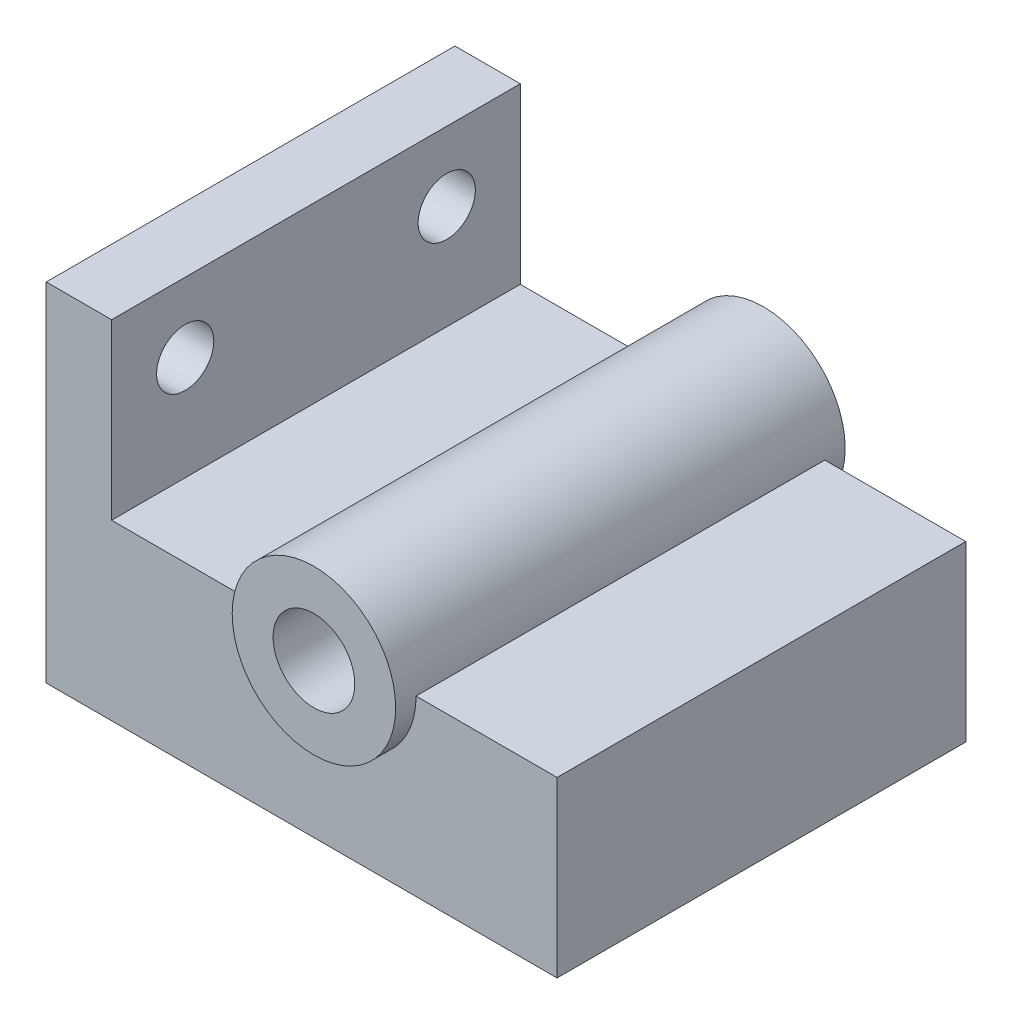
ISO-10303-21;
HEADER;
FILE_DESCRIPTION(('STEP AP214'),'2;1');
FILE_NAME('part.step','',(''),(''),'','','');
FILE_SCHEMA(('AUTOMOTIVE_DESIGN { 1 0 10303 214 1 1 1 1 }'));
ENDSEC;
DATA;
#1=APPLICATION_CONTEXT('core data for automotive mechanical design processes');
#2=APPLICATION_PROTOCOL_DEFINITION('international standard','automotive_design',2000,#1);
#3=PRODUCT_CONTEXT('',#1,'mechanical');
#4=PRODUCT('Part','Part','',(#3));
#5=PRODUCT_RELATED_PRODUCT_CATEGORY('part','',(#4));
#6=PRODUCT_DEFINITION_FORMATION('','',#4);
#7=PRODUCT_DEFINITION_CONTEXT('part definition',#1,'design');
#8=PRODUCT_DEFINITION('design','',#6,#7);
#9=PRODUCT_DEFINITION_SHAPE('','',#8);
#10=(LENGTH_UNIT() NAMED_UNIT(*) SI_UNIT(.MILLI.,.METRE.));
#11=(NAMED_UNIT(*) PLANE_ANGLE_UNIT() SI_UNIT($,.RADIAN.));
#12=(NAMED_UNIT(*) SI_UNIT($,.STERADIAN.) SOLID_ANGLE_UNIT());
#13=UNCERTAINTY_MEASURE_WITH_UNIT(LENGTH_MEASURE(1.E-05),#10,'distance_accuracy_value','');
#14=(GEOMETRIC_REPRESENTATION_CONTEXT(3) GLOBAL_UNCERTAINTY_ASSIGNED_CONTEXT((#13)) GLOBAL_UNIT_ASSIGNED_CONTEXT((#10,
#11,#12)) REPRESENTATION_CONTEXT('',''));
#15=CARTESIAN_POINT('',(0.,0.,0.));
#16=DIRECTION('',(0.,0.,1.));
#17=DIRECTION('',(1.,0.,0.));
#18=AXIS2_PLACEMENT_3D('',#15,#16,#17);
#19=CARTESIAN_POINT('',(125.,42.5,-100.));
#20=DIRECTION('',(0.,1.,0.));
#21=DIRECTION('',(-1.,0.,0.));
#22=AXIS2_PLACEMENT_3D('',#19,#20,#21);
#23=PLANE('',#22);
#24=DIRECTION('',(0.,0.,1.));
#25=VECTOR('',#24,1.);
#26=CARTESIAN_POINT('',(50.5,42.5,-100.));
#27=LINE('',#26,#25);
#28=CARTESIAN_POINT('',(50.5,42.5,-100.));
#29=VERTEX_POINT('',#28);
#30=CARTESIAN_POINT('',(50.5,42.5,0.));
#31=VERTEX_POINT('',#30);
#32=EDGE_CURVE('E122',#29,#31,#27,.T.);
#33=ORIENTED_EDGE('',*,*,#32,.F.);
#34=DIRECTION('',(-1.,0.,0.));
#35=VECTOR('',#34,1.);
#36=CARTESIAN_POINT('',(125.,42.5,-100.));
#37=LINE('',#36,#35);
#38=CARTESIAN_POINT('',(16.,42.5,-100.));
#39=VERTEX_POINT('',#38);
#40=EDGE_CURVE('E113',#29,#39,#37,.T.);
#41=ORIENTED_EDGE('',*,*,#40,.T.);
#42=DIRECTION('',(0.,0.,1.));
#43=VECTOR('',#42,1.);
#44=CARTESIAN_POINT('',(16.,42.5,-100.));
#45=LINE('',#44,#43);
#46=CARTESIAN_POINT('',(16.,42.5,0.));
#47=VERTEX_POINT('',#46);
#48=EDGE_CURVE('E117',#39,#47,#45,.T.);
#49=ORIENTED_EDGE('',*,*,#48,.T.);
#50=DIRECTION('',(-1.,0.,0.));
#51=VECTOR('',#50,1.);
#52=CARTESIAN_POINT('',(125.,42.5,0.));
#53=LINE('',#52,#51);
#54=EDGE_CURVE('E154',#31,#47,#53,.T.);
#55=ORIENTED_EDGE('',*,*,#54,.F.);
#56=EDGE_LOOP('',(#33,#41,#49,#55));
#57=FACE_BOUND('',#56,.T.);
#58=ADVANCED_FACE('F44',(#57),#23,.T.);
#59=CARTESIAN_POINT('',(0.,0.,-100.));
#60=DIRECTION('',(-1.,0.,0.));
#61=DIRECTION('',(0.,0.,1.));
#62=AXIS2_PLACEMENT_3D('',#59,#60,#61);
#63=PLANE('',#62);
#64=CARTESIAN_POINT('',(0.,68.,-18.));
#65=DIRECTION('',(-1.,0.,0.));
#66=DIRECTION('',(0.,0.,1.));
#67=AXIS2_PLACEMENT_3D('',#64,#65,#66);
#68=CIRCLE('',#67,7.00000000000001);
#69=CARTESIAN_POINT('',(0.,68.,-11.));
#70=VERTEX_POINT('',#69);
#71=EDGE_CURVE('E149',#70,#70,#68,.T.);
#72=ORIENTED_EDGE('',*,*,#71,.F.);
#73=EDGE_LOOP('',(#72));
#74=FACE_BOUND('',#73,.T.);
#75=CARTESIAN_POINT('',(0.,68.,-82.));
#76=DIRECTION('',(-1.,0.,0.));
#77=DIRECTION('',(0.,0.,1.));
#78=AXIS2_PLACEMENT_3D('',#75,#76,#77);
#79=CIRCLE('',#78,7.);
#80=CARTESIAN_POINT('',(0.,68.,-75.));
#81=VERTEX_POINT('',#80);
#82=EDGE_CURVE('E214',#81,#81,#79,.T.);
#83=ORIENTED_EDGE('',*,*,#82,.F.);
#84=EDGE_LOOP('',(#83));
#85=FACE_BOUND('',#84,.T.);
#86=DIRECTION('',(0.,-1.,0.));
#87=VECTOR('',#86,1.);
#88=CARTESIAN_POINT('',(0.,0.,0.));
#89=LINE('',#88,#87);
#90=CARTESIAN_POINT('',(0.,85.,0.));
#91=VERTEX_POINT('',#90);
#92=CARTESIAN_POINT('',(0.,0.,0.));
#93=VERTEX_POINT('',#92);
#94=EDGE_CURVE('E144',#91,#93,#89,.T.);
#95=ORIENTED_EDGE('',*,*,#94,.F.);
#96=DIRECTION('',(0.,0.,1.));
#97=VECTOR('',#96,1.);
#98=CARTESIAN_POINT('',(0.,85.,-100.));
#99=LINE('',#98,#97);
#100=CARTESIAN_POINT('',(0.,85.,-100.));
#101=VERTEX_POINT('',#100);
#102=EDGE_CURVE('E68',#101,#91,#99,.T.);
#103=ORIENTED_EDGE('',*,*,#102,.F.);
#104=DIRECTION('',(0.,-1.,0.));
#105=VECTOR('',#104,1.);
#106=CARTESIAN_POINT('',(0.,0.,-100.));
#107=LINE('',#106,#105);
#108=CARTESIAN_POINT('',(0.,0.,-100.));
#109=VERTEX_POINT('',#108);
#110=EDGE_CURVE('E165',#101,#109,#107,.T.);
#111=ORIENTED_EDGE('',*,*,#110,.T.);
#112=DIRECTION('',(0.,0.,1.));
#113=VECTOR('',#112,1.);
#114=CARTESIAN_POINT('',(0.,0.,-100.));
#115=LINE('',#114,#113);
#116=EDGE_CURVE('E47',#109,#93,#115,.T.);
#117=ORIENTED_EDGE('',*,*,#116,.T.);
#118=EDGE_LOOP('',(#95,#103,#111,#117));
#119=FACE_BOUND('',#118,.T.);
#120=ADVANCED_FACE('F50',(#74,#85,#119),#63,.T.);
#121=CARTESIAN_POINT('',(0.,85.,-100.));
#122=DIRECTION('',(0.,1.,0.));
#123=DIRECTION('',(0.,0.,1.));
#124=AXIS2_PLACEMENT_3D('',#121,#122,#123);
#125=PLANE('',#124);
#126=DIRECTION('',(-1.,0.,0.));
#127=VECTOR('',#126,1.);
#128=CARTESIAN_POINT('',(0.,85.,0.));
#129=LINE('',#128,#127);
#130=CARTESIAN_POINT('',(16.,85.,0.));
#131=VERTEX_POINT('',#130);
#132=EDGE_CURVE('E157',#131,#91,#129,.T.);
#133=ORIENTED_EDGE('',*,*,#132,.F.);
#134=DIRECTION('',(0.,0.,1.));
#135=VECTOR('',#134,1.);
#136=CARTESIAN_POINT('',(16.,85.,-100.));
#137=LINE('',#136,#135);
#138=CARTESIAN_POINT('',(16.,85.,-100.));
#139=VERTEX_POINT('',#138);
#140=EDGE_CURVE('E134',#139,#131,#137,.T.);
#141=ORIENTED_EDGE('',*,*,#140,.F.);
#142=DIRECTION('',(-1.,0.,0.));
#143=VECTOR('',#142,1.);
#144=CARTESIAN_POINT('',(0.,85.,-100.));
#145=LINE('',#144,#143);
#146=EDGE_CURVE('E136',#139,#101,#145,.T.);
#147=ORIENTED_EDGE('',*,*,#146,.T.);
#148=ORIENTED_EDGE('',*,*,#102,.T.);
#149=EDGE_LOOP('',(#133,#141,#147,#148));
#150=FACE_BOUND('',#149,.T.);
#151=ADVANCED_FACE('F166',(#150),#125,.T.);
#152=CARTESIAN_POINT('',(16.,85.,-100.));
#153=DIRECTION('',(1.,0.,0.));
#154=DIRECTION('',(0.,0.,-1.));
#155=AXIS2_PLACEMENT_3D('',#152,#153,#154);
#156=PLANE('',#155);
#157=CARTESIAN_POINT('',(16.,68.,-18.));
#158=DIRECTION('',(1.,0.,0.));
#159=DIRECTION('',(0.,0.,-1.));
#160=AXIS2_PLACEMENT_3D('',#157,#158,#159);
#161=CIRCLE('',#160,7.00000000000001);
#162=CARTESIAN_POINT('',(16.,68.,-25.));
#163=VERTEX_POINT('',#162);
#164=EDGE_CURVE('E215',#163,#163,#161,.T.);
#165=ORIENTED_EDGE('',*,*,#164,.F.);
#166=EDGE_LOOP('',(#165));
#167=FACE_BOUND('',#166,.T.);
#168=CARTESIAN_POINT('',(16.,68.,-82.));
#169=DIRECTION('',(1.,0.,0.));
#170=DIRECTION('',(0.,0.,-1.));
#171=AXIS2_PLACEMENT_3D('',#168,#169,#170);
#172=CIRCLE('',#171,7.);
#173=CARTESIAN_POINT('',(16.,68.,-89.));
#174=VERTEX_POINT('',#173);
#175=EDGE_CURVE('E211',#174,#174,#172,.T.);
#176=ORIENTED_EDGE('',*,*,#175,.F.);
#177=EDGE_LOOP('',(#176));
#178=FACE_BOUND('',#177,.T.);
#179=DIRECTION('',(0.,1.,0.));
#180=VECTOR('',#179,1.);
#181=CARTESIAN_POINT('',(16.,85.,0.));
#182=LINE('',#181,#180);
#183=EDGE_CURVE('E133',#47,#131,#182,.T.);
#184=ORIENTED_EDGE('',*,*,#183,.F.);
#185=ORIENTED_EDGE('',*,*,#48,.F.);
#186=DIRECTION('',(0.,1.,0.));
#187=VECTOR('',#186,1.);
#188=CARTESIAN_POINT('',(16.,85.,-100.));
#189=LINE('',#188,#187);
#190=EDGE_CURVE('E131',#39,#139,#189,.T.);
#191=ORIENTED_EDGE('',*,*,#190,.T.);
#192=ORIENTED_EDGE('',*,*,#140,.T.);
#193=EDGE_LOOP('',(#184,#185,#191,#192));
#194=FACE_BOUND('',#193,.T.);
#195=ADVANCED_FACE('F128',(#167,#178,#194),#156,.T.);
#196=DIRECTION('',(0.,0.,1.));
#197=VECTOR('',#196,1.);
#198=CARTESIAN_POINT('',(90.5,42.5,-100.));
#199=LINE('',#198,#197);
#200=CARTESIAN_POINT('',(90.5,42.5,0.));
#201=VERTEX_POINT('',#200);
#202=CARTESIAN_POINT('',(90.5,42.5,-100.));
#203=VERTEX_POINT('',#202);
#204=EDGE_CURVE('E199',#201,#203,#199,.F.);
#205=ORIENTED_EDGE('',*,*,#204,.F.);
#206=CARTESIAN_POINT('',(125.,42.5,0.));
#207=VERTEX_POINT('',#206);
#208=EDGE_CURVE('E156',#207,#201,#53,.T.);
#209=ORIENTED_EDGE('',*,*,#208,.F.);
#210=DIRECTION('',(0.,0.,1.));
#211=VECTOR('',#210,1.);
#212=CARTESIAN_POINT('',(125.,42.5,-100.));
#213=LINE('',#212,#211);
#214=CARTESIAN_POINT('',(125.,42.5,-100.));
#215=VERTEX_POINT('',#214);
#216=EDGE_CURVE('E137',#215,#207,#213,.T.);
#217=ORIENTED_EDGE('',*,*,#216,.F.);
#218=EDGE_CURVE('E123',#215,#203,#37,.T.);
#219=ORIENTED_EDGE('',*,*,#218,.T.);
#220=EDGE_LOOP('',(#205,#209,#217,#219));
#221=FACE_BOUND('',#220,.T.);
#222=ADVANCED_FACE('F177',(#221),#23,.T.);
#223=CARTESIAN_POINT('',(125.,0.,-100.));
#224=DIRECTION('',(1.,0.,0.));
#225=DIRECTION('',(0.,0.,-1.));
#226=AXIS2_PLACEMENT_3D('',#223,#224,#225);
#227=PLANE('',#226);
#228=DIRECTION('',(0.,1.,0.));
#229=VECTOR('',#228,1.);
#230=CARTESIAN_POINT('',(125.,0.,0.));
#231=LINE('',#230,#229);
#232=CARTESIAN_POINT('',(125.,0.,0.));
#233=VERTEX_POINT('',#232);
#234=EDGE_CURVE('E155',#233,#207,#231,.T.);
#235=ORIENTED_EDGE('',*,*,#234,.F.);
#236=DIRECTION('',(0.,0.,1.));
#237=VECTOR('',#236,1.);
#238=CARTESIAN_POINT('',(125.,0.,-100.));
#239=LINE('',#238,#237);
#240=CARTESIAN_POINT('',(125.,0.,-100.));
#241=VERTEX_POINT('',#240);
#242=EDGE_CURVE('E164',#241,#233,#239,.T.);
#243=ORIENTED_EDGE('',*,*,#242,.F.);
#244=DIRECTION('',(0.,1.,0.));
#245=VECTOR('',#244,1.);
#246=CARTESIAN_POINT('',(125.,0.,-100.));
#247=LINE('',#246,#245);
#248=EDGE_CURVE('E127',#241,#215,#247,.T.);
#249=ORIENTED_EDGE('',*,*,#248,.T.);
#250=ORIENTED_EDGE('',*,*,#216,.T.);
#251=EDGE_LOOP('',(#235,#243,#249,#250));
#252=FACE_BOUND('',#251,.T.);
#253=ADVANCED_FACE('F189',(#252),#227,.T.);
#254=CARTESIAN_POINT('',(0.,0.,-100.));
#255=DIRECTION('',(0.,-1.,0.));
#256=DIRECTION('',(0.,0.,-1.));
#257=AXIS2_PLACEMENT_3D('',#254,#255,#256);
#258=PLANE('',#257);
#259=DIRECTION('',(1.,0.,0.));
#260=VECTOR('',#259,1.);
#261=CARTESIAN_POINT('',(0.,0.,0.));
#262=LINE('',#261,#260);
#263=EDGE_CURVE('E146',#93,#233,#262,.T.);
#264=ORIENTED_EDGE('',*,*,#263,.F.);
#265=ORIENTED_EDGE('',*,*,#116,.F.);
#266=DIRECTION('',(1.,0.,0.));
#267=VECTOR('',#266,1.);
#268=CARTESIAN_POINT('',(0.,0.,-100.));
#269=LINE('',#268,#267);
#270=EDGE_CURVE('E224',#109,#241,#269,.T.);
#271=ORIENTED_EDGE('',*,*,#270,.T.);
#272=ORIENTED_EDGE('',*,*,#242,.T.);
#273=EDGE_LOOP('',(#264,#265,#271,#272));
#274=FACE_BOUND('',#273,.T.);
#275=ADVANCED_FACE('F170',(#274),#258,.T.);
#276=CARTESIAN_POINT('',(0.,0.,-100.));
#277=DIRECTION('',(0.,0.,-1.));
#278=DIRECTION('',(-1.,0.,0.));
#279=AXIS2_PLACEMENT_3D('',#276,#277,#278);
#280=PLANE('',#279);
#281=CARTESIAN_POINT('',(70.5,42.5,-100.));
#282=DIRECTION('',(0.,0.,-1.));
#283=DIRECTION('',(-1.,0.,0.));
#284=AXIS2_PLACEMENT_3D('',#281,#282,#283);
#285=CIRCLE('',#284,20.);
#286=EDGE_CURVE('E11',#203,#29,#285,.T.);
#287=ORIENTED_EDGE('',*,*,#286,.F.);
#288=ORIENTED_EDGE('',*,*,#218,.F.);
#289=ORIENTED_EDGE('',*,*,#248,.F.);
#290=ORIENTED_EDGE('',*,*,#270,.F.);
#291=ORIENTED_EDGE('',*,*,#110,.F.);
#292=ORIENTED_EDGE('',*,*,#146,.F.);
#293=ORIENTED_EDGE('',*,*,#190,.F.);
#294=ORIENTED_EDGE('',*,*,#40,.F.);
#295=EDGE_LOOP('',(#287,#288,#289,#290,#291,#292,#293,#294));
#296=FACE_BOUND('',#295,.T.);
#297=ADVANCED_FACE('F140',(#296),#280,.T.);
#298=CARTESIAN_POINT('',(0.,0.,0.));
#299=DIRECTION('',(0.,0.,-1.));
#300=DIRECTION('',(-1.,0.,0.));
#301=AXIS2_PLACEMENT_3D('',#298,#299,#300);
#302=PLANE('',#301);
#303=CARTESIAN_POINT('',(70.5,42.5,0.));
#304=DIRECTION('',(0.,0.,1.));
#305=DIRECTION('',(1.,0.,0.));
#306=AXIS2_PLACEMENT_3D('',#303,#304,#305);
#307=CIRCLE('',#306,20.);
#308=EDGE_CURVE('E53',#31,#201,#307,.T.);
#309=ORIENTED_EDGE('',*,*,#308,.F.);
#310=ORIENTED_EDGE('',*,*,#54,.T.);
#311=ORIENTED_EDGE('',*,*,#183,.T.);
#312=ORIENTED_EDGE('',*,*,#132,.T.);
#313=ORIENTED_EDGE('',*,*,#94,.T.);
#314=ORIENTED_EDGE('',*,*,#263,.T.);
#315=ORIENTED_EDGE('',*,*,#234,.T.);
#316=ORIENTED_EDGE('',*,*,#208,.T.);
#317=EDGE_LOOP('',(#309,#310,#311,#312,#313,#314,#315,#316));
#318=FACE_BOUND('',#317,.T.);
#319=ADVANCED_FACE('F169',(#318),#302,.F.);
#320=CARTESIAN_POINT('',(-84.,68.,-82.));
#321=DIRECTION('',(1.,0.,0.));
#322=DIRECTION('',(0.,0.,-1.));
#323=AXIS2_PLACEMENT_3D('',#320,#321,#322);
#324=CYLINDRICAL_SURFACE('',#323,7.);
#325=ORIENTED_EDGE('',*,*,#82,.T.);
#326=EDGE_LOOP('',(#325));
#327=FACE_BOUND('',#326,.T.);
#328=ORIENTED_EDGE('',*,*,#175,.T.);
#329=EDGE_LOOP('',(#328));
#330=FACE_BOUND('',#329,.T.);
#331=ADVANCED_FACE('F231',(#327,#330),#324,.F.);
#332=CARTESIAN_POINT('',(-84.,68.,-18.));
#333=DIRECTION('',(1.,0.,0.));
#334=DIRECTION('',(0.,0.,-1.));
#335=AXIS2_PLACEMENT_3D('',#332,#333,#334);
#336=CYLINDRICAL_SURFACE('',#335,7.00000000000001);
#337=ORIENTED_EDGE('',*,*,#71,.T.);
#338=EDGE_LOOP('',(#337));
#339=FACE_BOUND('',#338,.T.);
#340=ORIENTED_EDGE('',*,*,#164,.T.);
#341=EDGE_LOOP('',(#340));
#342=FACE_BOUND('',#341,.T.);
#343=ADVANCED_FACE('F228',(#339,#342),#336,.F.);
#344=CARTESIAN_POINT('',(70.5,42.5,-100.));
#345=DIRECTION('',(0.,0.,1.));
#346=DIRECTION('',(1.,0.,0.));
#347=AXIS2_PLACEMENT_3D('',#344,#345,#346);
#348=CYLINDRICAL_SURFACE('',#347,20.);
#349=ORIENTED_EDGE('',*,*,#204,.T.);
#350=ORIENTED_EDGE('',*,*,#286,.T.);
#351=ORIENTED_EDGE('',*,*,#32,.T.);
#352=ORIENTED_EDGE('',*,*,#308,.T.);
#353=EDGE_LOOP('',(#349,#350,#351,#352));
#354=FACE_BOUND('',#353,.T.);
#355=CARTESIAN_POINT('',(70.5,42.5,5.));
#356=DIRECTION('',(0.,0.,1.));
#357=DIRECTION('',(1.,0.,0.));
#358=AXIS2_PLACEMENT_3D('',#355,#356,#357);
#359=CIRCLE('',#358,20.);
#360=CARTESIAN_POINT('',(90.5,42.5,5.));
#361=VERTEX_POINT('',#360);
#362=EDGE_CURVE('E201',#361,#361,#359,.T.);
#363=ORIENTED_EDGE('',*,*,#362,.F.);
#364=EDGE_LOOP('',(#363));
#365=FACE_BOUND('',#364,.T.);
#366=CARTESIAN_POINT('',(70.5,42.5,-105.));
#367=DIRECTION('',(0.,0.,-1.));
#368=DIRECTION('',(-1.,0.,0.));
#369=AXIS2_PLACEMENT_3D('',#366,#367,#368);
#370=CIRCLE('',#369,20.);
#371=CARTESIAN_POINT('',(50.5,42.5,-105.));
#372=VERTEX_POINT('',#371);
#373=EDGE_CURVE('E384',#372,#372,#370,.T.);
#374=ORIENTED_EDGE('',*,*,#373,.F.);
#375=EDGE_LOOP('',(#374));
#376=FACE_BOUND('',#375,.T.);
#377=ADVANCED_FACE('F202',(#354,#365,#376),#348,.T.);
#378=CARTESIAN_POINT('',(70.5,42.5,5.));
#379=DIRECTION('',(0.,0.,1.));
#380=DIRECTION('',(1.,0.,0.));
#381=AXIS2_PLACEMENT_3D('',#378,#379,#380);
#382=PLANE('',#381);
#383=CARTESIAN_POINT('',(70.5,42.5,4.99999999999999));
#384=DIRECTION('',(0.,0.,-1.));
#385=DIRECTION('',(-1.,0.,0.));
#386=AXIS2_PLACEMENT_3D('',#383,#384,#385);
#387=CIRCLE('',#386,10.);
#388=CARTESIAN_POINT('',(60.5,42.5,4.99999999999999));
#389=VERTEX_POINT('',#388);
#390=EDGE_CURVE('E379',#389,#389,#387,.T.);
#391=ORIENTED_EDGE('',*,*,#390,.T.);
#392=EDGE_LOOP('',(#391));
#393=FACE_BOUND('',#392,.T.);
#394=ORIENTED_EDGE('',*,*,#362,.T.);
#395=EDGE_LOOP('',(#394));
#396=FACE_BOUND('',#395,.T.);
#397=ADVANCED_FACE('F286',(#393,#396),#382,.T.);
#398=CARTESIAN_POINT('',(70.5,42.5,-105.));
#399=DIRECTION('',(0.,0.,-1.));
#400=DIRECTION('',(-1.,0.,0.));
#401=AXIS2_PLACEMENT_3D('',#398,#399,#400);
#402=PLANE('',#401);
#403=CARTESIAN_POINT('',(70.5,42.5,-105.));
#404=DIRECTION('',(0.,0.,-1.));
#405=DIRECTION('',(-1.,0.,0.));
#406=AXIS2_PLACEMENT_3D('',#403,#404,#405);
#407=CIRCLE('',#406,10.);
#408=CARTESIAN_POINT('',(60.5,42.5,-105.));
#409=VERTEX_POINT('',#408);
#410=EDGE_CURVE('E382',#409,#409,#407,.T.);
#411=ORIENTED_EDGE('',*,*,#410,.F.);
#412=EDGE_LOOP('',(#411));
#413=FACE_BOUND('',#412,.T.);
#414=ORIENTED_EDGE('',*,*,#373,.T.);
#415=EDGE_LOOP('',(#414));
#416=FACE_BOUND('',#415,.T.);
#417=ADVANCED_FACE('F300',(#413,#416),#402,.T.);
#418=CARTESIAN_POINT('',(70.5,42.5,4.99999999999999));
#419=DIRECTION('',(0.,0.,-1.));
#420=DIRECTION('',(-1.,0.,0.));
#421=AXIS2_PLACEMENT_3D('',#418,#419,#420);
#422=CYLINDRICAL_SURFACE('',#421,10.);
#423=ORIENTED_EDGE('',*,*,#390,.F.);
#424=EDGE_LOOP('',(#423));
#425=FACE_BOUND('',#424,.T.);
#426=ORIENTED_EDGE('',*,*,#410,.T.);
#427=EDGE_LOOP('',(#426));
#428=FACE_BOUND('',#427,.T.);
#429=ADVANCED_FACE('F307',(#425,#428),#422,.F.);
#430=CLOSED_SHELL('',(#58,#120,#151,#195,#222,#253,#275,#297,#319,#331,#343,#377,#397,#417,#429));
#431=MANIFOLD_SOLID_BREP('B2',#430);
#432=ADVANCED_BREP_SHAPE_REPRESENTATION('',(#18,#431),#14);
#433=SHAPE_DEFINITION_REPRESENTATION(#9,#432);
ENDSEC;
END-ISO-10303-21;
